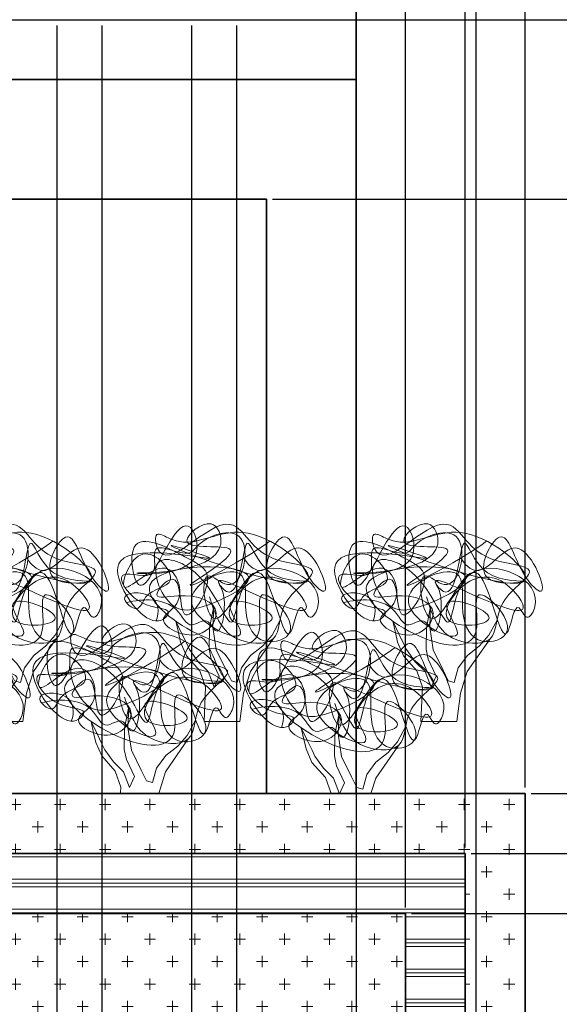
# Model space of a CAD drawing. Units: millimetres. Extents: x -692 to 9639, y -141 to 10345.
# Tile 8 of 19: x 7929 to 8831, y 1504 to 3148. Entities that reach past the tile are written whole.
import ezdxf

# ---------------------------------------------------------------- set-up
doc = ezdxf.new("R2010")
doc.units = ezdxf.units.MM
doc.header["$MEASUREMENT"] = 0
for name, color, linetype, lineweight in [('A-ANNO-DIMS', 2, 'Continuous', 18), ('A-ELEV', 7, 'Continuous', 35), ('A-ELEV-PATT', 8, 'Continuous', 13), ('L-PLNT', 3, 'Continuous', 18)]:
    doc.layers.add(name, color=color, linetype=linetype, lineweight=lineweight)
doc.styles.get("Standard").update_dxf_attribs({"font": 'arial.ttf'})
doc.dimstyles.get("Standard").update_dxf_attribs({"dimtxt": 25, "dimasz": 20, "dimexe": 0.18, "dimexo": 10, "dimgap": 10, "dimtad": 0, "dimtih": 1, "dimtoh": 1, "dimdec": 0, "dimzin": 0, "dimdsep": 46, "dimtxsty": 'Standard', "dimcen": 10, "dimadec": 0, "dimazin": 0, "dimtfac": 1, "dimtdec": 0, "dimtofl": 0, "dimtmove": 0, "dimatfit": 3, "dimfxl": 1, "dimtolj": 1, "dimtzin": 0, "dimarcsym": 0})

# ---------------------------------------------------------------- blocks, each defined once
blk = doc.blocks.new('SHRUB-A')
for p, q in [((56.2, 156.7), (63.1, 192.4)), ((63.1, 192.4), (61.6, 157.6)), ((4.3, 148.6), (0, 167.6)), ((0, 167.6), (10, 146.8)), ((160.6, 144.2), (174.3, 169.5)), ((7.9, 132.5), (4.3, 148.6)), ((55.6, 120.9), (56.2, 156.7)), ((61.6, 157.6), (67.3, 119.6)), ((17.8, 109.9), (7.9, 132.5)), ((10, 146.8), (18, 130.3)), ((162.4, 138.4), (124.4, 83.7)), ((145.1, 126.5), (160.6, 144.2)), ((18, 130.3), (22.9, 120.3)), ((22.9, 120.3), (37.4, 100.1)), ((59.1, 104.1), (55.6, 120.9)), ((67.3, 119.6), (83.9, 86)), ((124.8, 110.5), (145.1, 126.5)), ((40.2, 84.8), (17.8, 109.9)), ((37.4, 100.1), (54, 83.6)), ((72.4, 75.8), (59.1, 104.1)), ((109.4, 89.7), (124.8, 110.5)), ((49.7, 57.7), (40.2, 84.8)), ((54, 83.6), (64.1, 57.4)), ((83.9, 86), (92.7, 68.2)), ((102.6, 65.4), (109.4, 89.7)), ((124.4, 83.7), (113, 47.4)), ((64.1, 57.4), (72.4, 75.8)), ((92.7, 68.2), (102.6, 65.4)), ((47, 0.4), (49.7, 57.7)), ((113, 47.4), (106.7, 0)), ((106.7, 0), (47, 0.4))]:
    blk.add_line(p, q)
blk = doc.blocks.new('SHRUB-B')
for p, q in [((56.2, 99.2), (63.1, 135)), ((63.1, 135), (61.6, 100.2)), ((4.3, 91.2), (0, 110.2)), ((0, 110.2), (10, 89.4)), ((55.6, 63.5), (56.2, 99.2)), ((61.6, 100.2), (67.3, 62.2)), ((160.6, 86.8), (174.3, 112.1)), ((7.9, 75.1), (4.3, 91.2)), ((10, 89.4), (18, 72.9)), ((145.1, 69.1), (160.6, 86.8)), ((17.8, 52.5), (7.9, 75.1)), ((18, 72.9), (22.9, 62.9)), ((124.8, 53.1), (145.1, 69.1)), ((40.2, 27.4), (17.8, 52.5)), ((22.9, 62.9), (37.4, 42.7)), ((59.1, 46.7), (55.6, 63.5)), ((67.3, 62.2), (83.9, 28.6)), ((109.4, 32.3), (124.8, 53.1)), ((37.4, 42.7), (54, 26.2)), ((72.4, 18.4), (59.1, 46.7)), ((49.7, 0.3), (40.2, 27.4)), ((54, 26.2), (64.1, 0)), ((64.1, 0), (72.4, 18.4)), ((83.9, 28.6), (92.7, 10.8)), ((102.6, 8), (109.4, 32.3)), ((92.7, 10.8), (102.6, 8))]:
    blk.add_line(p, q)
blk = doc.blocks.new('*D7')
at = {"layer": 'A-ANNO-DIMS', "color": 0, "lineweight": -2, "transparency": 16777216}
for p, q in [((8481.5, 9848.8), (-649.1, 9848.8)), ((-648.9, 9828.8), (-648.9, 5124.9)), ((-648.9, 375.6), (-648.9, 5079.4)), ((2463.7, 355.6), (-649.1, 355.6))]:
    blk.add_line(p, q, dxfattribs=at)
at = {"layer": 'A-ANNO-DIMS', "color": 0, "lineweight": -3, "transparency": 16777216}
for points in [[(-652.2, 9828.8), (-645.6, 9828.8), (-648.9, 9848.8)], [(-652.2, 375.6), (-645.6, 375.6), (-648.9, 355.6)]]:
    blk.add_solid(points, dxfattribs=at)
at = {"layer": 'Defpoints', "color": 0, "lineweight": -3, "transparency": 16777216}
for p in [(-648.9, 9848.8), (8491.5, 9848.8), (2473.7, 355.6)]:
    blk.add_point(p, dxfattribs=at)
at = {"layer": 'A-ANNO-DIMS', "color": 0, "transparency": 16777216, "insert": (-648.9, 5102.2), "char_height": 25, "attachment_point": 5}
blk.add_mtext('\\A1;9493', dxfattribs=at)
blk = doc.blocks.new('*D9')
at = {"layer": 'A-ANNO-DIMS', "color": 0, "lineweight": -2, "transparency": 16777216}
for p, q in [((8501.5, 8848.8), (9553.9, 8848.8)), ((9553.7, 8828.8), (9553.7, 4874.9)), ((9553.7, 875.6), (9553.7, 4829.4)), ((9083.7, 855.6), (9553.9, 855.6))]:
    blk.add_line(p, q, dxfattribs=at)
at = {"layer": 'A-ANNO-DIMS', "color": 0, "lineweight": -3, "transparency": 16777216}
for points in [[(9550.4, 8828.8), (9557.1, 8828.8), (9553.7, 8848.8)], [(9550.4, 875.6), (9557.1, 875.6), (9553.7, 855.6)]]:
    blk.add_solid(points, dxfattribs=at)
at = {"layer": 'Defpoints', "color": 0, "lineweight": -3, "transparency": 16777216}
for p in [(8491.5, 8848.8), (9553.7, 8848.8), (9073.7, 855.6)]:
    blk.add_point(p, dxfattribs=at)
at = {"layer": 'A-ANNO-DIMS', "color": 0, "transparency": 16777216, "insert": (9553.7, 4852.2), "char_height": 25, "attachment_point": 5}
blk.add_mtext('\\A1;7993', dxfattribs=at)
blk = doc.blocks.new('*D28')
at = {"layer": 'A-ANNO-DIMS', "color": 0, "lineweight": -2, "transparency": 16777216}
for p, q in [((8583.7, 1655.6), (9553.9, 1655.6)), ((9553.7, 1635.6), (9553.7, 1278.3)), ((9553.7, 875.6), (9553.7, 1232.8)), ((8583.7, 855.6), (9553.9, 855.6))]:
    blk.add_line(p, q, dxfattribs=at)
at = {"layer": 'A-ANNO-DIMS', "color": 0, "lineweight": -3, "transparency": 16777216}
for points in [[(9550.4, 1635.6), (9557.1, 1635.6), (9553.7, 1655.6)], [(9550.4, 875.6), (9557.1, 875.6), (9553.7, 855.6)]]:
    blk.add_solid(points, dxfattribs=at)
at = {"layer": 'Defpoints', "color": 0, "lineweight": -3, "transparency": 16777216}
for p in [(8573.7, 1655.6), (9553.7, 1655.6), (8573.7, 855.6)]:
    blk.add_point(p, dxfattribs=at)
at = {"layer": 'A-ANNO-DIMS', "color": 0, "transparency": 16777216, "insert": (9553.7, 1255.6), "char_height": 25, "attachment_point": 5}
blk.add_mtext('\\A1;800', dxfattribs=at)
blk = doc.blocks.new('*D29')
at = {"layer": 'A-ANNO-DIMS', "color": 0, "lineweight": -2, "transparency": 16777216}
for p, q in [((9553.7, 1755.6), (9553.7, 1775.6)), ((9553.7, 1775.6), (9573.7, 1775.6)), ((8683.7, 1755.6), (9553.9, 1755.6)), ((9553.7, 1675.6), (9553.7, 1735.6)), ((8583.7, 1655.6), (9553.9, 1655.6))]:
    blk.add_line(p, q, dxfattribs=at)
at = {"layer": 'A-ANNO-DIMS', "color": 0, "lineweight": -3, "transparency": 16777216}
for points in [[(9550.4, 1735.6), (9557.1, 1735.6), (9553.7, 1755.6)], [(9550.4, 1675.6), (9557.1, 1675.6), (9553.7, 1655.6)]]:
    blk.add_solid(points, dxfattribs=at)
at = {"layer": 'Defpoints', "color": 0, "lineweight": -3, "transparency": 16777216}
for p in [(8673.7, 1755.6), (9553.7, 1755.6), (8573.7, 1655.6)]:
    blk.add_point(p, dxfattribs=at)
at = {"layer": 'A-ANNO-DIMS', "color": 0, "transparency": 16777216, "insert": (9610.1, 1775.6), "char_height": 25, "attachment_point": 5}
blk.add_mtext('\\A1;100', dxfattribs=at)
blk = doc.blocks.new('*D30')
at = {"layer": 'A-ANNO-DIMS', "color": 0, "lineweight": -2, "transparency": 16777216}
for p, q in [((9553.7, 1855.6), (9553.7, 1875.6)), ((9553.7, 1875.6), (9573.7, 1875.6)), ((8783.7, 1855.6), (9553.9, 1855.6)), ((9553.7, 1775.6), (9553.7, 1835.6)), ((8683.7, 1755.6), (9553.9, 1755.6))]:
    blk.add_line(p, q, dxfattribs=at)
at = {"layer": 'A-ANNO-DIMS', "color": 0, "lineweight": -3, "transparency": 16777216}
for points in [[(9550.4, 1835.6), (9557.1, 1835.6), (9553.7, 1855.6)], [(9550.4, 1775.6), (9557.1, 1775.6), (9553.7, 1755.6)]]:
    blk.add_solid(points, dxfattribs=at)
at = {"layer": 'Defpoints', "color": 0, "lineweight": -3, "transparency": 16777216}
for p in [(8773.7, 1855.6), (9553.7, 1855.6), (8673.7, 1755.6)]:
    blk.add_point(p, dxfattribs=at)
at = {"layer": 'A-ANNO-DIMS', "color": 0, "transparency": 16777216, "insert": (9610.1, 1875.6), "char_height": 25, "attachment_point": 5}
blk.add_mtext('\\A1;100', dxfattribs=at)
blk = doc.blocks.new('*D31')
at = {"layer": 'A-ANNO-DIMS', "color": 0, "lineweight": -2, "transparency": 16777216}
for p, q in [((8351.5, 2848.3), (9553.9, 2848.3)), ((9553.7, 2828.3), (9553.7, 2374.7)), ((9553.7, 1875.6), (9553.7, 2329.2)), ((8783.7, 1855.6), (9553.9, 1855.6))]:
    blk.add_line(p, q, dxfattribs=at)
at = {"layer": 'A-ANNO-DIMS', "color": 0, "lineweight": -3, "transparency": 16777216}
for points in [[(9550.4, 2828.3), (9557.1, 2828.3), (9553.7, 2848.3)], [(9550.4, 1875.6), (9557.1, 1875.6), (9553.7, 1855.6)]]:
    blk.add_solid(points, dxfattribs=at)
at = {"layer": 'Defpoints', "color": 0, "lineweight": -3, "transparency": 16777216}
for p in [(8341.5, 2848.3), (9553.7, 2848.3), (8773.7, 1855.6)]:
    blk.add_point(p, dxfattribs=at)
at = {"layer": 'A-ANNO-DIMS', "color": 0, "transparency": 16777216, "insert": (9553.7, 2351.9), "char_height": 25, "attachment_point": 5}
blk.add_mtext('\\A1;992.7', dxfattribs=at)
blk = doc.blocks.new('*D34')
at = {"layer": 'A-ANNO-DIMS', "color": 0, "lineweight": -2, "transparency": 16777216}
for p, q in [((7091.7, 1665.6), (7091.7, 10329)), ((7111.7, 10328.8), (7786.7, 10328.8)), ((8553.7, 10328.8), (7878.8, 10328.8)), ((8573.7, 1665.6), (8573.7, 10329))]:
    blk.add_line(p, q, dxfattribs=at)
at = {"layer": 'A-ANNO-DIMS', "color": 0, "lineweight": -3, "transparency": 16777216}
for points in [[(7111.7, 10332.1), (7111.7, 10325.4), (7091.7, 10328.8)], [(8553.7, 10332.1), (8553.7, 10325.4), (8573.7, 10328.8)]]:
    blk.add_solid(points, dxfattribs=at)
at = {"layer": 'Defpoints', "color": 0, "lineweight": -3, "transparency": 16777216}
for p in [(8573.7, 10328.8), (7091.7, 1655.6), (8573.7, 1655.6)]:
    blk.add_point(p, dxfattribs=at)
at = {"layer": 'A-ANNO-DIMS', "color": 0, "transparency": 16777216, "insert": (7832.7, 10328.8), "char_height": 25, "attachment_point": 5}
blk.add_mtext('\\A1;1482', dxfattribs=at)
blk = doc.blocks.new('*D35')
at = {"layer": 'A-ANNO-DIMS', "color": 0, "lineweight": -2, "transparency": 16777216}
for p, q in [((8553.7, 10328.8), (8533.7, 10328.8)), ((8573.7, 1665.6), (8573.7, 10329)), ((8673.7, 1765.6), (8673.7, 10329)), ((8693.7, 10328.8), (8713.7, 10328.8))]:
    blk.add_line(p, q, dxfattribs=at)
at = {"layer": 'A-ANNO-DIMS', "color": 0, "lineweight": -3, "transparency": 16777216}
for points in [[(8553.7, 10332.1), (8553.7, 10325.4), (8573.7, 10328.8)], [(8693.7, 10332.1), (8693.7, 10325.4), (8673.7, 10328.8)]]:
    blk.add_solid(points, dxfattribs=at)
at = {"layer": 'Defpoints', "color": 0, "lineweight": -3, "transparency": 16777216}
for p in [(8673.7, 10328.8), (8673.7, 1755.6), (8573.7, 1655.6)]:
    blk.add_point(p, dxfattribs=at)
at = {"layer": 'A-ANNO-DIMS', "color": 0, "transparency": 16777216, "insert": (8623.7, 10328.8), "char_height": 25, "attachment_point": 5}
blk.add_mtext('\\A1;100', dxfattribs=at)
blk = doc.blocks.new('*D36')
at = {"layer": 'A-ANNO-DIMS', "color": 0, "lineweight": -2, "transparency": 16777216}
for p, q in [((8653.7, 10328.8), (8633.7, 10328.8)), ((8673.7, 1765.6), (8673.7, 10329)), ((8773.7, 1865.6), (8773.7, 10329)), ((8793.7, 10328.8), (8813.7, 10328.8))]:
    blk.add_line(p, q, dxfattribs=at)
at = {"layer": 'A-ANNO-DIMS', "color": 0, "lineweight": -3, "transparency": 16777216}
for points in [[(8653.7, 10332.1), (8653.7, 10325.4), (8673.7, 10328.8)], [(8793.7, 10332.1), (8793.7, 10325.4), (8773.7, 10328.8)]]:
    blk.add_solid(points, dxfattribs=at)
at = {"layer": 'Defpoints', "color": 0, "lineweight": -3, "transparency": 16777216}
for p in [(8773.7, 10328.8), (8773.7, 1855.6), (8673.7, 1755.6)]:
    blk.add_point(p, dxfattribs=at)
at = {"layer": 'A-ANNO-DIMS', "color": 0, "transparency": 16777216, "insert": (8723.7, 10328.8), "char_height": 25, "attachment_point": 5}
blk.add_mtext('\\A1;100', dxfattribs=at)
blk = doc.blocks.new('*D46')
at = {"layer": 'A-ANNO-DIMS', "color": 0, "lineweight": -2, "transparency": 16777216}
for p, q in [((7841.5, 3138.3), (7841.5, -124.6)), ((7991.5, 3138.3), (7991.5, -124.6)), ((7861.5, -124.4), (7880.1, -124.4)), ((7971.5, -124.4), (7952.9, -124.4))]:
    blk.add_line(p, q, dxfattribs=at)
at = {"layer": 'A-ANNO-DIMS', "color": 0, "lineweight": -3, "transparency": 16777216}
for points in [[(7861.5, -121.1), (7861.5, -127.8), (7841.5, -124.4)], [(7971.5, -121.1), (7971.5, -127.8), (7991.5, -124.4)]]:
    blk.add_solid(points, dxfattribs=at)
at = {"layer": 'Defpoints', "color": 0, "lineweight": -3, "transparency": 16777216}
for p in [(7841.5, 3148.3), (7991.5, 3148.3), (7991.5, -124.4)]:
    blk.add_point(p, dxfattribs=at)
at = {"layer": 'A-ANNO-DIMS', "color": 0, "transparency": 16777216, "insert": (7916.5, -124.4), "char_height": 25, "attachment_point": 5}
blk.add_mtext('\\A1;150', dxfattribs=at)
blk = doc.blocks.new('*D47')
at = {"layer": 'A-ANNO-DIMS', "color": 0, "lineweight": -2, "transparency": 16777216}
for p, q in [((7991.5, 3138.3), (7991.5, -124.6)), ((8066.5, 3138.3), (8066.5, -124.6)), ((8011.5, -124.4), (8046.5, -124.4)), ((8066.5, -124.4), (8086.5, -124.4))]:
    blk.add_line(p, q, dxfattribs=at)
at = {"layer": 'A-ANNO-DIMS', "color": 0, "lineweight": -3, "transparency": 16777216}
for points in [[(8011.5, -121.1), (8011.5, -127.8), (7991.5, -124.4)], [(8046.5, -121.1), (8046.5, -127.8), (8066.5, -124.4)]]:
    blk.add_solid(points, dxfattribs=at)
at = {"layer": 'Defpoints', "color": 0, "lineweight": -3, "transparency": 16777216}
for p in [(7991.5, 3148.3), (8066.5, 3148.3), (8066.5, -124.4)]:
    blk.add_point(p, dxfattribs=at)
at = {"layer": 'A-ANNO-DIMS', "color": 0, "transparency": 16777216, "insert": (8114.4, -124.4), "char_height": 25, "attachment_point": 5}
blk.add_mtext('\\A1;75', dxfattribs=at)
blk = doc.blocks.new('*D48')
at = {"layer": 'A-ANNO-DIMS', "color": 0, "lineweight": -2, "transparency": 16777216}
for p, q in [((8066.5, 3138.3), (8066.5, -124.6)), ((8216.5, 3138.3), (8216.5, -124.6)), ((8086.5, -124.4), (8105.1, -124.4)), ((8196.5, -124.4), (8177.9, -124.4))]:
    blk.add_line(p, q, dxfattribs=at)
at = {"layer": 'A-ANNO-DIMS', "color": 0, "lineweight": -3, "transparency": 16777216}
for points in [[(8086.5, -121.1), (8086.5, -127.8), (8066.5, -124.4)], [(8196.5, -121.1), (8196.5, -127.8), (8216.5, -124.4)]]:
    blk.add_solid(points, dxfattribs=at)
at = {"layer": 'Defpoints', "color": 0, "lineweight": -3, "transparency": 16777216}
for p in [(8066.5, 3148.3), (8216.5, 3148.3), (8216.5, -124.4)]:
    blk.add_point(p, dxfattribs=at)
at = {"layer": 'A-ANNO-DIMS', "color": 0, "transparency": 16777216, "insert": (8141.5, -124.4), "char_height": 25, "attachment_point": 5}
blk.add_mtext('\\A1;150', dxfattribs=at)
blk = doc.blocks.new('*D49')
at = {"layer": 'A-ANNO-DIMS', "color": 0, "lineweight": -2, "transparency": 16777216}
for p, q in [((8216.5, 3138.3), (8216.5, -124.6)), ((8291.5, 3138.3), (8291.5, -124.6)), ((8236.5, -124.4), (8271.5, -124.4)), ((8291.5, -124.4), (8311.5, -124.4))]:
    blk.add_line(p, q, dxfattribs=at)
at = {"layer": 'A-ANNO-DIMS', "color": 0, "lineweight": -3, "transparency": 16777216}
for points in [[(8236.5, -121.1), (8236.5, -127.8), (8216.5, -124.4)], [(8271.5, -121.1), (8271.5, -127.8), (8291.5, -124.4)]]:
    blk.add_solid(points, dxfattribs=at)
at = {"layer": 'Defpoints', "color": 0, "lineweight": -3, "transparency": 16777216}
for p in [(8216.5, 3148.3), (8291.5, 3148.3), (8291.5, -124.4)]:
    blk.add_point(p, dxfattribs=at)
at = {"layer": 'A-ANNO-DIMS', "color": 0, "transparency": 16777216, "insert": (8339.4, -124.4), "char_height": 25, "attachment_point": 5}
blk.add_mtext('\\A1;75', dxfattribs=at)
blk = doc.blocks.new('*D50')
at = {"layer": 'A-ANNO-DIMS', "color": 0, "lineweight": -2, "transparency": 16777216}
for p, q in [((8291.5, 3138.3), (8291.5, -124.6)), ((8491.5, 3138.3), (8491.5, -124.6)), ((8311.5, -124.4), (8353.8, -124.4)), ((8471.5, -124.4), (8429.3, -124.4))]:
    blk.add_line(p, q, dxfattribs=at)
at = {"layer": 'A-ANNO-DIMS', "color": 0, "lineweight": -3, "transparency": 16777216}
for points in [[(8311.5, -121.1), (8311.5, -127.8), (8291.5, -124.4)], [(8471.5, -121.1), (8471.5, -127.8), (8491.5, -124.4)]]:
    blk.add_solid(points, dxfattribs=at)
at = {"layer": 'Defpoints', "color": 0, "lineweight": -3, "transparency": 16777216}
for p in [(8291.5, 3148.3), (8491.5, 3148.3), (8491.5, -124.4)]:
    blk.add_point(p, dxfattribs=at)
at = {"layer": 'A-ANNO-DIMS', "color": 0, "transparency": 16777216, "insert": (8391.5, -124.4), "char_height": 25, "attachment_point": 5}
blk.add_mtext('\\A1;200', dxfattribs=at)
blk = doc.blocks.new('*D51')
at = {"layer": 'A-ANNO-DIMS', "color": 0, "lineweight": -2, "transparency": 16777216}
for p, q in [((8691.5, 4838.8), (8691.5, -124.6)), ((8491.5, 3138.3), (8491.5, -124.6)), ((8511.5, -124.4), (8553.8, -124.4)), ((8671.5, -124.4), (8629.3, -124.4))]:
    blk.add_line(p, q, dxfattribs=at)
at = {"layer": 'A-ANNO-DIMS', "color": 0, "lineweight": -3, "transparency": 16777216}
for points in [[(8511.5, -121.1), (8511.5, -127.8), (8491.5, -124.4)], [(8671.5, -121.1), (8671.5, -127.8), (8691.5, -124.4)]]:
    blk.add_solid(points, dxfattribs=at)
at = {"layer": 'Defpoints', "color": 0, "lineweight": -3, "transparency": 16777216}
for p in [(8691.5, 4848.8), (8491.5, 3148.3), (8691.5, -124.4)]:
    blk.add_point(p, dxfattribs=at)
at = {"layer": 'A-ANNO-DIMS', "color": 0, "transparency": 16777216, "insert": (8591.5, -124.4), "char_height": 25, "attachment_point": 5}
blk.add_mtext('\\A1;200', dxfattribs=at)
blk = doc.blocks.new('*D71')
at = {"layer": 'A-ANNO-DIMS', "color": 0, "lineweight": -2, "transparency": 16777216}
for p, q in [((5201.5, 3598.3), (9553.9, 3598.3)), ((9553.7, 3578.3), (9553.7, 3396)), ((9553.7, 3168.3), (9553.7, 3350.5)), ((5101.5, 3148.3), (9553.9, 3148.3))]:
    blk.add_line(p, q, dxfattribs=at)
at = {"layer": 'A-ANNO-DIMS', "color": 0, "lineweight": -3, "transparency": 16777216}
for points in [[(9550.4, 3578.3), (9557.1, 3578.3), (9553.7, 3598.3)], [(9550.4, 3168.3), (9557.1, 3168.3), (9553.7, 3148.3)]]:
    blk.add_solid(points, dxfattribs=at)
at = {"layer": 'Defpoints', "color": 0, "lineweight": -3, "transparency": 16777216}
for p in [(5191.5, 3598.3), (9553.7, 3598.3), (5091.5, 3148.3)]:
    blk.add_point(p, dxfattribs=at)
at = {"layer": 'A-ANNO-DIMS', "color": 0, "transparency": 16777216, "insert": (9553.7, 3373.3), "char_height": 25, "attachment_point": 5}
blk.add_mtext('\\A1;450', dxfattribs=at)

msp = doc.modelspace()

# ---------------------------------------------------------------- hatches: boundary and pattern name
at = {"layer": 'A-ELEV-PATT'}
h = msp.add_hatch(dxfattribs=at)
h.set_pattern_fill('CROSS', color=256, scale=150)
h.paths.add_polyline_path([(8573.746, 1655.575), (7091.746, 1655.575), (7091.746, 855.575), (7273.746, 855.575), (8573.746, 855.575)], flags=17)
h.paths.add_polyline_path([(8773.746, 1855.575), (8463.966, 1855.575), (8463.828, 1855.268), (8463.709, 1855.575), (7761.103, 1855.575), (7760.965, 1855.268), (7760.846, 1855.575), (7409.705, 1855.575), (7409.567, 1855.268), (7409.448, 1855.575), (7076.174, 1855.575), (7076.035, 1855.268), (7075.916, 1855.575), (6891.746, 1855.575), (6891.746, 855.575), (6991.746, 855.575), (6991.746, 1755.575), (8673.746, 1755.575), (8673.746, 855.575), (8773.746, 855.575)])
h = msp.add_hatch(dxfattribs=at)
h.set_pattern_fill('PLAST', color=256, scale=200)
h.paths.add_polyline_path([(8673.746, 1755.575), (6991.746, 1755.575), (6991.746, 855.575), (7091.746, 855.575), (7091.746, 1655.575), (8573.746, 1655.575), (8573.746, 855.575), (8673.746, 855.575)])

# ---------------------------------------------------------------- linework, layer by layer
at = {"layer": 'A-ELEV'}
for p, q in [((8491.547, 4848.772), (8491.547, 1855.575)), ((5191.547, 3048.27), (8491.547, 3048.27)), ((5773.746, 2848.27), (8341.547, 2848.27)), ((8341.547, 2848.27), (8341.547, 1855.575)), ((8773.746, 1855.575), (6891.746, 1855.575)), ((8773.746, 1855.575), (8773.746, 855.575)), ((8673.746, 1755.575), (6991.746, 1755.575)), ((8673.746, 1755.575), (8673.746, 855.575)), ((8573.746, 1655.575), (7091.746, 1655.575)), ((8573.746, 1655.575), (8573.746, 855.575))]:
    msp.add_line(p, q, dxfattribs=at)
at = {"layer": 'L-PLNT'}
for p, q in [((8104.579, 1965.211), (8111.567, 2000.918)), ((8111.567, 2000.918), (8110.002, 1966.165)), ((8052.702, 1957.134), (8048.428, 1976.125)), ((8048.428, 1976.125), (8058.469, 1955.382)), ((8208.984, 1952.778), (8222.715, 1978.029)), ((8056.315, 1941.086), (8052.702, 1957.134)), ((8104.023, 1929.473), (8104.579, 1965.211)), ((8110.002, 1966.165), (8115.774, 1928.138)), ((8066.226, 1918.461), (8056.315, 1941.086)), ((8058.469, 1955.382), (8066.458, 1938.88)), ((8210.873, 1946.937), (8172.808, 1892.206)), ((8193.491, 1935.076), (8208.984, 1952.778)), ((8066.458, 1938.88), (8071.29, 1928.899)), ((8071.29, 1928.899), (8085.863, 1908.658)), ((8107.495, 1912.661), (8104.023, 1929.473)), ((8115.774, 1928.138), (8132.332, 1894.515)), ((8173.193, 1919.065), (8193.491, 1935.076)), ((8562.132, 1936.243), (8524.067, 1881.512)), ((8088.612, 1893.382), (8066.226, 1918.461)), ((8085.863, 1908.658), (8102.421, 1892.113)), ((8120.848, 1884.375), (8107.495, 1912.661)), ((8157.83, 1898.301), (8173.193, 1919.065)), ((8098.109, 1866.269), (8088.612, 1893.382)), ((8102.421, 1892.113), (8112.569, 1865.962)), ((8132.332, 1894.515), (8141.082, 1876.748)), ((8151.027, 1873.967), (8157.83, 1898.301)), ((8172.808, 1892.206), (8161.459, 1856.004)), ((8112.569, 1865.962), (8120.848, 1884.375)), ((8141.082, 1876.748), (8151.027, 1873.967)), ((8524.067, 1881.512), (8516.49, 1857.344)), ((8097.695, 1857.344), (8098.109, 1866.269))]:
    msp.add_line(p, q, dxfattribs=at)
for points, knots in [([(7941.428, 2249.042), (7947.933, 2237.706), (7981.169, 2207.754), (8037.599, 2319.362), (8096.779, 2167.67), (8032.143, 2229.166), (8016.418, 2328.371), (7949.459, 2194.758), (8086.925, 2215.079), (7970.08, 2204.712), (7940.744, 2329.754), (7935.142, 2163.076), (7882.64, 2224.979), (7976.321, 2179.391), (8073.386, 2141.303), (8004.226, 2230.619), (7938.072, 2210.89), (7895.861, 2127.262), (8046.749, 2141.658), (7881.14, 2203.471), (7977.514, 2083.661), (7783.672, 2177.336), (7958.368, 2256.385), (7936.159, 2158.211), (7964.897, 2098.948), (8051.149, 2123.83), (7949.315, 2228.342), (8004.521, 2029.162), (7618.927, 2240.289), (8034.021, 2243.554), (7884.038, 2166.62), (7813.186, 2156.226), (7770.374, 2264.065), (7885.155, 2230.339), (7927.243, 2085.9), (7932.228, 2275.464), (8093.922, 2209.432), (8051.195, 2140.066), (8033.158, 2187.643), (8012.363, 2051.748), (7975.609, 2333.663), (7888.478, 2070.375), (7863.476, 2246.68), (7933.245, 2175.732), (7964.912, 2316.142), (7874.371, 2285.782), (7845.246, 2244.752), (7778.303, 2291.151), (7804.494, 2204.577), (7712.052, 2240.713), (7761.869, 2161.604), (7823.388, 2165.76), (7793.222, 2127.131), (7737.918, 2181.977), (7713.636, 2288.868), (7958.01, 2226.655), (7709.719, 2307.83), (8170.468, 2128.857), (7944.803, 2328.1), (7864.96, 2267.378), (7818.657, 2280.064), (7790.573, 2295.919), (7802.935, 2206.055), (7904.263, 2346.33), (7956.403, 2266.58), (7995.218, 2241.096), (8086.893, 2233.207), (7993.877, 2180.878), (8008.037, 2100.111), (7908.22, 2108.211), (7892.593, 2156.893), (7883.85, 2184.132)], [2413.81083439, 2413.81083439, 2413.81083439, 2413.81083439, 2446.13175162, 2525.76080664, 2606.35842411, 2641.00152553, 2720.74212251, 2790.99014926, 2851.81652626, 2913.32865241, 2976.26621652, 3063.90114016, 3082.75198237, 3142.42040078, 3234.21047015, 3290.89514405, 3366.44484787, 3415.98940505, 3483.69911772, 3557.93307926, 3609.73318023, 3705.73947781, 3799.4035149, 3865.9559372, 3923.0506034, 3967.47996902, 4044.49288828, 4106.44083814, 4304.51898163, 4470.20683119, 4567.66187689, 4605.3795614, 4686.71522755, 4750.59418277, 4853.67923318, 4940.38216709, 5061.92671957, 5081.75583403, 5102.38342504, 5145.20608443, 5257.20859169, 5364.77120979, 5434.601162, 5468.93345211, 5548.91442162, 5624.29444335, 5636.24531967, 5696.20028889, 5735.53268567, 5783.76480276, 5846.42206129, 5886.03768999, 5892.5373904, 5975.51315878, 6025.10951571, 6171.93373357, 6229.50952465, 6457.88730992, 6585.61219414, 6694.59236697, 6720.94216912, 6740.48817363, 6762.80712224, 6890.45590486, 6938.76737224, 6996.52597549, 7050.2147859, 7119.04318667, 7183.57042671, 7247.02609863, 7327.63038966, 7327.63038966, 7327.63038966, 7327.63038966]), ([(7794.737, 2143.94), (7800.8, 2158.144), (7797.305, 2196.249), (7722.734, 2191.386), (7766.182, 2154.108), (7776.863, 2198.183), (7845.924, 2201.259), (7765.972, 2293.571), (7717.477, 2156.7), (7815.952, 2271.959), (7847.727, 2174.361), (7783.674, 2143.553), (7866.477, 2102.288), (7913.823, 2169.843), (7849.377, 2193.667), (7778.836, 2176.214), (7840.34, 2245.325), (7827.395, 2104.492), (7901.707, 2221.171), (7835.943, 2254.125), (7740.167, 2308.243), (7764.333, 2163.685), (7803.906, 2260.33), (7851.043, 2324.908), (7884.633, 2215.034), (7655.885, 2230.018), (7930.034, 2217.011), (7890.032, 2326.244), (7806.634, 2255.543), (7981.668, 2284.242), (7770.144, 2159.222), (7934.397, 2239.906), (7984.529, 2277.481)], [369.05069933, 369.05069933, 369.05069933, 369.05069933, 408.0755152, 451.81999766, 477.70991819, 501.76804774, 551.72688153, 614.71506468, 677.59190345, 752.65992621, 814.92518896, 848.06947292, 911.78367098, 957.89252981, 1028.01014559, 1063.15062915, 1099.93333455, 1162.00574744, 1235.23981988, 1278.45742209, 1371.86548038, 1434.47491944, 1513.90135623, 1562.79289697, 1613.81915843, 1716.27616866, 1864.9556669, 1902.31221643, 1951.61463942, 2025.20033993, 2111.30740148, 2244.75178922, 2244.75178922, 2244.75178922, 2244.75178922]), ([(8303.871, 2249.042), (8310.377, 2237.706), (8343.613, 2207.754), (8400.043, 2319.362), (8459.223, 2167.67), (8394.587, 2229.166), (8378.861, 2328.371), (8311.902, 2194.758), (8449.368, 2215.079), (8332.524, 2204.712), (8303.188, 2329.754), (8297.585, 2163.076), (8245.084, 2224.979), (8338.764, 2179.391), (8435.83, 2141.303), (8366.669, 2230.619), (8300.516, 2210.89), (8258.305, 2127.262), (8409.192, 2141.658), (8243.583, 2203.471), (8339.958, 2083.661), (8146.116, 2177.336), (8320.812, 2256.385), (8298.603, 2158.211), (8327.34, 2098.948), (8413.593, 2123.83), (8311.759, 2228.342), (8366.965, 2029.162), (7981.371, 2240.289), (8396.465, 2243.554), (8246.482, 2166.62), (8175.63, 2156.226), (8132.817, 2264.065), (8247.598, 2230.339), (8289.686, 2085.9), (8294.672, 2275.464), (8456.365, 2209.432), (8413.638, 2140.066), (8395.601, 2187.643), (8374.806, 2051.748), (8338.053, 2333.663), (8250.921, 2070.375), (8225.919, 2246.68), (8295.688, 2175.732), (8327.355, 2316.142), (8236.815, 2285.782), (8207.689, 2244.752), (8140.747, 2291.151), (8166.938, 2204.577), (8074.496, 2240.713), (8124.312, 2161.604), (8185.832, 2165.76), (8155.665, 2127.131), (8100.361, 2181.977), (8076.08, 2288.868), (8320.454, 2226.655), (8072.162, 2307.83), (8532.911, 2128.857), (8307.247, 2328.1), (8227.403, 2267.378), (8181.101, 2280.064), (8153.017, 2295.919), (8165.379, 2206.055), (8266.707, 2346.33), (8318.847, 2266.58), (8357.661, 2241.096), (8449.337, 2233.207), (8356.32, 2180.878), (8370.481, 2100.111), (8270.663, 2108.211), (8255.037, 2156.893), (8246.293, 2184.132)], [2413.81083439, 2413.81083439, 2413.81083439, 2413.81083439, 2446.13175162, 2525.76080664, 2606.35842411, 2641.00152553, 2720.74212251, 2790.99014926, 2851.81652626, 2913.32865241, 2976.26621652, 3063.90114016, 3082.75198237, 3142.42040078, 3234.21047015, 3290.89514405, 3366.44484787, 3415.98940505, 3483.69911772, 3557.93307926, 3609.73318023, 3705.73947781, 3799.4035149, 3865.9559372, 3923.0506034, 3967.47996902, 4044.49288828, 4106.44083814, 4304.51898163, 4470.20683119, 4567.66187689, 4605.3795614, 4686.71522755, 4750.59418277, 4853.67923318, 4940.38216709, 5061.92671957, 5081.75583403, 5102.38342504, 5145.20608443, 5257.20859169, 5364.77120979, 5434.601162, 5468.93345211, 5548.91442162, 5624.29444335, 5636.24531967, 5696.20028889, 5735.53268567, 5783.76480276, 5846.42206129, 5886.03768999, 5892.5373904, 5975.51315878, 6025.10951571, 6171.93373357, 6229.50952465, 6457.88730992, 6585.61219414, 6694.59236697, 6720.94216912, 6740.48817363, 6762.80712224, 6890.45590486, 6938.76737224, 6996.52597549, 7050.2147859, 7119.04318667, 7183.57042671, 7247.02609863, 7327.63038966, 7327.63038966, 7327.63038966, 7327.63038966]), ([(8157.18, 2143.94), (8163.243, 2158.144), (8159.749, 2196.249), (8085.177, 2191.386), (8128.625, 2154.108), (8139.307, 2198.183), (8208.368, 2201.259), (8128.416, 2293.571), (8079.92, 2156.7), (8178.396, 2271.959), (8210.171, 2174.361), (8146.118, 2143.553), (8228.92, 2102.288), (8276.267, 2169.843), (8211.821, 2193.667), (8141.279, 2176.214), (8202.784, 2245.325), (8189.839, 2104.492), (8264.151, 2221.171), (8198.387, 2254.125), (8102.611, 2308.243), (8126.776, 2163.685), (8166.35, 2260.33), (8213.486, 2324.908), (8247.077, 2215.034), (8018.329, 2230.018), (8292.478, 2217.011), (8252.476, 2326.244), (8169.077, 2255.543), (8344.112, 2284.242), (8132.588, 2159.222), (8296.841, 2239.906), (8346.972, 2277.481)], [369.05069933, 369.05069933, 369.05069933, 369.05069933, 408.0755152, 451.81999766, 477.70991819, 501.76804774, 551.72688153, 614.71506468, 677.59190345, 752.65992621, 814.92518896, 848.06947292, 911.78367098, 957.89252981, 1028.01014559, 1063.15062915, 1099.93333455, 1162.00574744, 1235.23981988, 1278.45742209, 1371.86548038, 1434.47491944, 1513.90135623, 1562.79289697, 1613.81915843, 1716.27616866, 1864.9556669, 1902.31221643, 1951.61463942, 2025.20033993, 2111.30740148, 2244.75178922, 2244.75178922, 2244.75178922, 2244.75178922]), ([(8666.315, 2249.042), (8672.821, 2237.706), (8706.056, 2207.754), (8762.486, 2319.362), (8821.667, 2167.67), (8757.03, 2229.166), (8741.305, 2328.371), (8674.346, 2194.758), (8811.812, 2215.079), (8694.967, 2204.712), (8665.631, 2329.754), (8660.029, 2163.076), (8607.527, 2224.979), (8701.208, 2179.391), (8798.274, 2141.303), (8729.113, 2230.619), (8662.959, 2210.89), (8620.748, 2127.262), (8771.636, 2141.658), (8606.027, 2203.471), (8702.401, 2083.661), (8508.559, 2177.336), (8683.255, 2256.385), (8661.047, 2158.211), (8689.784, 2098.948), (8776.036, 2123.83), (8674.202, 2228.342), (8729.408, 2029.162), (8343.815, 2240.289), (8758.908, 2243.554), (8608.925, 2166.62), (8538.073, 2156.226), (8495.261, 2264.065), (8610.042, 2230.339), (8652.13, 2085.9), (8657.115, 2275.464), (8818.809, 2209.432), (8776.082, 2140.066), (8758.045, 2187.643), (8737.25, 2051.748), (8700.496, 2333.663), (8613.365, 2070.375), (8588.363, 2246.68), (8658.132, 2175.732), (8689.799, 2316.142), (8599.258, 2285.782), (8570.133, 2244.752), (8503.19, 2291.151), (8529.381, 2204.577), (8436.939, 2240.713), (8486.756, 2161.604), (8548.276, 2165.76), (8518.109, 2127.131), (8462.805, 2181.977), (8438.523, 2288.868), (8682.898, 2226.655), (8434.606, 2307.83), (8895.355, 2128.857), (8669.69, 2328.1), (8589.847, 2267.378), (8543.544, 2280.064), (8515.46, 2295.919), (8527.822, 2206.055), (8629.151, 2346.33), (8681.29, 2266.58), (8720.105, 2241.096), (8811.781, 2233.207), (8718.764, 2180.878), (8732.925, 2100.111), (8633.107, 2108.211), (8617.48, 2156.893), (8608.737, 2184.132)], [2413.81083439, 2413.81083439, 2413.81083439, 2413.81083439, 2446.13175162, 2525.76080664, 2606.35842411, 2641.00152553, 2720.74212251, 2790.99014926, 2851.81652626, 2913.32865241, 2976.26621652, 3063.90114016, 3082.75198237, 3142.42040078, 3234.21047015, 3290.89514405, 3366.44484787, 3415.98940505, 3483.69911772, 3557.93307926, 3609.73318023, 3705.73947781, 3799.4035149, 3865.9559372, 3923.0506034, 3967.47996902, 4044.49288828, 4106.44083814, 4304.51898163, 4470.20683119, 4567.66187689, 4605.3795614, 4686.71522755, 4750.59418277, 4853.67923318, 4940.38216709, 5061.92671957, 5081.75583403, 5102.38342504, 5145.20608443, 5257.20859169, 5364.77120979, 5434.601162, 5468.93345211, 5548.91442162, 5624.29444335, 5636.24531967, 5696.20028889, 5735.53268567, 5783.76480276, 5846.42206129, 5886.03768999, 5892.5373904, 5975.51315878, 6025.10951571, 6171.93373357, 6229.50952465, 6457.88730992, 6585.61219414, 6694.59236697, 6720.94216912, 6740.48817363, 6762.80712224, 6890.45590486, 6938.76737224, 6996.52597549, 7050.2147859, 7119.04318667, 7183.57042671, 7247.02609863, 7327.63038966, 7327.63038966, 7327.63038966, 7327.63038966]), ([(8519.624, 2143.94), (8525.687, 2158.144), (8522.192, 2196.249), (8447.621, 2191.386), (8491.069, 2154.108), (8501.75, 2198.183), (8570.811, 2201.259), (8490.859, 2293.571), (8442.364, 2156.7), (8540.839, 2271.959), (8572.615, 2174.361), (8508.561, 2143.553), (8591.364, 2102.288), (8638.711, 2169.843), (8574.264, 2193.667), (8503.723, 2176.214), (8565.227, 2245.325), (8552.283, 2104.492), (8626.594, 2221.171), (8560.83, 2254.125), (8465.055, 2308.243), (8489.22, 2163.685), (8528.793, 2260.33), (8575.93, 2324.908), (8609.521, 2215.034), (8380.773, 2230.018), (8654.921, 2217.011), (8614.92, 2326.244), (8531.521, 2255.543), (8706.555, 2284.242), (8495.031, 2159.222), (8659.285, 2239.906), (8709.416, 2277.481)], [369.05069933, 369.05069933, 369.05069933, 369.05069933, 408.0755152, 451.81999766, 477.70991819, 501.76804774, 551.72688153, 614.71506468, 677.59190345, 752.65992621, 814.92518896, 848.06947292, 911.78367098, 957.89252981, 1028.01014559, 1063.15062915, 1099.93333455, 1162.00574744, 1235.23981988, 1278.45742209, 1371.86548038, 1434.47491944, 1513.90135623, 1562.79289697, 1613.81915843, 1716.27616866, 1864.9556669, 1902.31221643, 1951.61463942, 2025.20033993, 2111.30740148, 2244.75178922, 2244.75178922, 2244.75178922, 2244.75178922]), ([(8261.901, 2206.874), (8265.391, 2200.207), (8276.888, 2178.247), (8263.817, 2104.319), (8242.636, 2153.752), (8209.825, 2125.304), (8192.239, 2181.552), (8134.486, 2182.208), (8107.774, 2174.344)], [0, 0, 0, 0, 24.87287104, 81.92705424, 103.09014331, 128.64171207, 165.87657864, 231.33124244, 231.33124244, 231.33124244, 231.33124244]), ([(8624.344, 2206.874), (8627.835, 2200.207), (8639.331, 2178.247), (8626.26, 2104.319), (8605.079, 2153.752), (8572.269, 2125.304), (8554.682, 2181.552), (8496.929, 2182.208), (8470.218, 2174.344)], [0, 0, 0, 0, 24.87287104, 81.92705424, 103.09014331, 128.64171207, 165.87657864, 231.33124244, 231.33124244, 231.33124244, 231.33124244]), ([(8162.096, 2081.693), (8168.601, 2070.358), (8201.837, 2040.406), (8258.267, 2152.014), (8317.447, 2000.321), (8252.811, 2061.817), (8237.086, 2161.023), (8170.127, 2027.41), (8307.593, 2047.73), (8190.748, 2037.363), (8161.412, 2162.405), (8155.81, 1995.728), (8103.308, 2057.63), (8196.989, 2012.042), (8294.055, 1973.955), (8224.894, 2063.27), (8158.74, 2043.541), (8116.529, 1959.913), (8267.417, 1974.309), (8101.808, 2036.122), (8198.182, 1916.312), (8004.34, 2009.987), (8179.036, 2089.036), (8156.828, 1990.863), (8185.565, 1931.599), (8271.817, 1956.482), (8169.983, 2060.993), (8225.189, 1861.813), (7839.595, 2072.94), (8254.689, 2076.205), (8104.706, 1999.271), (8033.854, 1988.878), (7991.042, 2096.717), (8105.823, 2062.99), (8147.911, 1918.551), (8152.896, 2108.116), (8314.59, 2042.083), (8271.863, 1972.717), (8253.826, 2020.295), (8233.031, 1884.399), (8196.277, 2166.314), (8109.146, 1903.027), (8084.144, 2079.331), (8153.913, 2008.384), (8185.58, 2148.793), (8095.039, 2118.434), (8065.914, 2077.403), (7998.971, 2123.803), (8025.162, 2037.228), (7932.72, 2073.364), (7982.537, 1994.255), (8044.056, 1998.412), (8013.89, 1959.783), (7958.586, 2014.628), (7934.304, 2121.519), (8178.679, 2059.306), (7930.387, 2140.481), (8391.136, 1961.508), (8165.471, 2160.751), (8085.628, 2100.029), (8039.325, 2112.716), (8011.241, 2128.571), (8023.603, 2038.706), (8124.932, 2178.981), (8177.071, 2099.231), (8215.886, 2073.747), (8307.562, 2065.858), (8214.545, 2013.53), (8228.705, 1932.762), (8128.888, 1940.862), (8113.261, 1989.545), (8104.518, 2016.783)], [2413.81083439, 2413.81083439, 2413.81083439, 2413.81083439, 2446.13175162, 2525.76080664, 2606.35842411, 2641.00152553, 2720.74212251, 2790.99014926, 2851.81652626, 2913.32865241, 2976.26621652, 3063.90114016, 3082.75198237, 3142.42040078, 3234.21047015, 3290.89514405, 3366.44484787, 3415.98940505, 3483.69911772, 3557.93307926, 3609.73318023, 3705.73947781, 3799.4035149, 3865.9559372, 3923.0506034, 3967.47996902, 4044.49288828, 4106.44083814, 4304.51898163, 4470.20683119, 4567.66187689, 4605.3795614, 4686.71522755, 4750.59418277, 4853.67923318, 4940.38216709, 5061.92671957, 5081.75583403, 5102.38342504, 5145.20608443, 5257.20859169, 5364.77120979, 5434.601162, 5468.93345211, 5548.91442162, 5624.29444335, 5636.24531967, 5696.20028889, 5735.53268567, 5783.76480276, 5846.42206129, 5886.03768999, 5892.5373904, 5975.51315878, 6025.10951571, 6171.93373357, 6229.50952465, 6457.88730992, 6585.61219414, 6694.59236697, 6720.94216912, 6740.48817363, 6762.80712224, 6890.45590486, 6938.76737224, 6996.52597549, 7050.2147859, 7119.04318667, 7183.57042671, 7247.02609863, 7327.63038966, 7327.63038966, 7327.63038966, 7327.63038966]), ([(8015.405, 1976.591), (8021.468, 1990.795), (8017.973, 2028.9), (7943.402, 2024.038), (7986.85, 1986.759), (7997.531, 2030.834), (8066.592, 2033.911), (7986.64, 2126.222), (7938.145, 1989.352), (8036.62, 2104.61), (8068.395, 2007.013), (8004.342, 1976.204), (8087.145, 1934.94), (8134.491, 2002.494), (8070.045, 2026.318), (7999.504, 2008.866), (8061.008, 2077.976), (8048.064, 1937.143), (8122.375, 2053.823), (8056.611, 2086.776), (7960.836, 2140.895), (7985.001, 1996.336), (8024.574, 2092.982), (8071.711, 2157.56), (8105.302, 2047.686), (7876.554, 2062.669), (8150.702, 2049.663), (8110.701, 2158.895), (8027.302, 2088.194), (8202.336, 2116.894), (7990.812, 1991.873), (8155.065, 2072.558), (8205.197, 2110.133)], [369.05069933, 369.05069933, 369.05069933, 369.05069933, 408.0755152, 451.81999766, 477.70991819, 501.76804774, 551.72688153, 614.71506468, 677.59190345, 752.65992621, 814.92518896, 848.06947292, 911.78367098, 957.89252981, 1028.01014559, 1063.15062915, 1099.93333455, 1162.00574744, 1235.23981988, 1278.45742209, 1371.86548038, 1434.47491944, 1513.90135623, 1562.79289697, 1613.81915843, 1716.27616866, 1864.9556669, 1902.31221643, 1951.61463942, 2025.20033993, 2111.30740148, 2244.75178922, 2244.75178922, 2244.75178922, 2244.75178922]), ([(7810.492, 2070.999), (7816.997, 2059.664), (7850.233, 2029.712), (7906.663, 2141.319), (7965.843, 1989.627), (7901.207, 2051.123), (7885.481, 2150.328), (7818.522, 2016.716), (7955.988, 2037.036), (7839.144, 2026.669), (7809.808, 2151.711), (7804.206, 1985.034), (7751.704, 2046.936), (7845.385, 2001.348), (7942.45, 1963.26), (7873.289, 2052.576), (7807.136, 2032.847), (7764.925, 1949.219), (7915.813, 1963.615), (7750.204, 2025.428), (7846.578, 1905.618), (7652.736, 1999.293), (7827.432, 2078.342), (7805.223, 1980.168), (7833.961, 1920.905), (7920.213, 1945.788), (7818.379, 2050.299), (7873.585, 1851.119), (7487.991, 2062.246), (7903.085, 2065.511), (7753.102, 1988.577), (7682.25, 1978.184), (7639.438, 2086.023), (7754.219, 2052.296), (7796.307, 1907.857), (7801.292, 2097.422), (7962.985, 2031.389), (7920.258, 1962.023), (7902.221, 2009.601), (7881.426, 1873.705), (7844.673, 2155.62), (7757.542, 1892.333), (7732.54, 2068.637), (7802.309, 1997.689), (7833.975, 2138.099), (7743.435, 2107.74), (7714.309, 2066.709), (7647.367, 2113.109), (7673.558, 2026.534), (7581.116, 2062.67), (7630.933, 1983.561), (7692.452, 1987.717), (7662.286, 1949.089), (7606.982, 2003.934), (7582.7, 2110.825), (7827.074, 2048.612), (7578.782, 2129.787), (8039.532, 1950.814), (7813.867, 2150.057), (7734.023, 2089.335), (7687.721, 2102.021), (7659.637, 2117.876), (7671.999, 2028.012), (7773.327, 2168.287), (7825.467, 2088.537), (7864.281, 2063.053), (7955.957, 2055.164), (7862.94, 2002.836), (7877.101, 1922.068), (7777.284, 1930.168), (7761.657, 1978.85), (7752.914, 2006.089)], [2413.81083439, 2413.81083439, 2413.81083439, 2413.81083439, 2446.13175162, 2525.76080664, 2606.35842411, 2641.00152553, 2720.74212251, 2790.99014926, 2851.81652626, 2913.32865241, 2976.26621652, 3063.90114016, 3082.75198237, 3142.42040078, 3234.21047015, 3290.89514405, 3366.44484787, 3415.98940505, 3483.69911772, 3557.93307926, 3609.73318023, 3705.73947781, 3799.4035149, 3865.9559372, 3923.0506034, 3967.47996902, 4044.49288828, 4106.44083814, 4304.51898163, 4470.20683119, 4567.66187689, 4605.3795614, 4686.71522755, 4750.59418277, 4853.67923318, 4940.38216709, 5061.92671957, 5081.75583403, 5102.38342504, 5145.20608443, 5257.20859169, 5364.77120979, 5434.601162, 5468.93345211, 5548.91442162, 5624.29444335, 5636.24531967, 5696.20028889, 5735.53268567, 5783.76480276, 5846.42206129, 5886.03768999, 5892.5373904, 5975.51315878, 6025.10951571, 6171.93373357, 6229.50952465, 6457.88730992, 6585.61219414, 6694.59236697, 6720.94216912, 6740.48817363, 6762.80712224, 6890.45590486, 6938.76737224, 6996.52597549, 7050.2147859, 7119.04318667, 7183.57042671, 7247.02609863, 7327.63038966, 7327.63038966, 7327.63038966, 7327.63038966]), ([(8513.355, 2070.999), (8519.86, 2059.664), (8553.096, 2029.712), (8609.526, 2141.319), (8668.706, 1989.627), (8604.07, 2051.123), (8588.345, 2150.328), (8521.386, 2016.716), (8658.852, 2037.036), (8542.007, 2026.669), (8512.671, 2151.711), (8507.069, 1985.034), (8454.567, 2046.936), (8548.248, 2001.348), (8645.313, 1963.26), (8576.153, 2052.576), (8509.999, 2032.847), (8467.788, 1949.219), (8618.676, 1963.615), (8453.067, 2025.428), (8549.441, 1905.618), (8355.599, 1999.293), (8530.295, 2078.342), (8508.086, 1980.168), (8536.824, 1920.905), (8623.076, 1945.788), (8521.242, 2050.299), (8576.448, 1851.119), (8190.854, 2062.246), (8605.948, 2065.511), (8455.965, 1988.577), (8385.113, 1978.184), (8342.301, 2086.023), (8457.082, 2052.296), (8499.17, 1907.857), (8504.155, 2097.422), (8665.849, 2031.389), (8623.122, 1962.023), (8605.084, 2009.601), (8584.29, 1873.705), (8547.536, 2155.62), (8460.405, 1892.333), (8435.403, 2068.637), (8505.172, 1997.689), (8536.839, 2138.099), (8446.298, 2107.74), (8417.172, 2066.709), (8350.23, 2113.109), (8376.421, 2026.534), (8283.979, 2062.67), (8333.796, 1983.561), (8395.315, 1987.717), (8365.149, 1949.089), (8309.845, 2003.934), (8285.563, 2110.825), (8529.937, 2048.612), (8281.646, 2129.787), (8742.395, 1950.814), (8516.73, 2150.057), (8436.887, 2089.335), (8390.584, 2102.021), (8362.5, 2117.876), (8374.862, 2028.012), (8476.19, 2168.287), (8528.33, 2088.537), (8567.145, 2063.053), (8658.82, 2055.164), (8565.804, 2002.836), (8579.964, 1922.068), (8480.147, 1930.168), (8464.52, 1978.85), (8455.777, 2006.089)], [2413.81083439, 2413.81083439, 2413.81083439, 2413.81083439, 2446.13175162, 2525.76080664, 2606.35842411, 2641.00152553, 2720.74212251, 2790.99014926, 2851.81652626, 2913.32865241, 2976.26621652, 3063.90114016, 3082.75198237, 3142.42040078, 3234.21047015, 3290.89514405, 3366.44484787, 3415.98940505, 3483.69911772, 3557.93307926, 3609.73318023, 3705.73947781, 3799.4035149, 3865.9559372, 3923.0506034, 3967.47996902, 4044.49288828, 4106.44083814, 4304.51898163, 4470.20683119, 4567.66187689, 4605.3795614, 4686.71522755, 4750.59418277, 4853.67923318, 4940.38216709, 5061.92671957, 5081.75583403, 5102.38342504, 5145.20608443, 5257.20859169, 5364.77120979, 5434.601162, 5468.93345211, 5548.91442162, 5624.29444335, 5636.24531967, 5696.20028889, 5735.53268567, 5783.76480276, 5846.42206129, 5886.03768999, 5892.5373904, 5975.51315878, 6025.10951571, 6171.93373357, 6229.50952465, 6457.88730992, 6585.61219414, 6694.59236697, 6720.94216912, 6740.48817363, 6762.80712224, 6890.45590486, 6938.76737224, 6996.52597549, 7050.2147859, 7119.04318667, 7183.57042671, 7247.02609863, 7327.63038966, 7327.63038966, 7327.63038966, 7327.63038966]), ([(8366.664, 1965.897), (8372.727, 1980.101), (8369.232, 2018.206), (8294.661, 2013.343), (8338.109, 1976.065), (8348.79, 2020.14), (8417.851, 2023.217), (8337.899, 2115.528), (8289.404, 1978.657), (8387.879, 2093.916), (8419.654, 1996.319), (8355.601, 1965.51), (8438.404, 1924.245), (8485.75, 1991.8), (8421.304, 2015.624), (8350.763, 1998.171), (8412.267, 2067.282), (8399.322, 1926.449), (8473.634, 2043.128), (8407.87, 2076.082), (8312.094, 2130.201), (8336.26, 1985.642), (8375.833, 2082.287), (8422.97, 2146.866), (8456.56, 2036.992), (8227.812, 2051.975), (8501.961, 2038.969), (8461.959, 2148.201), (8378.56, 2077.5), (8553.595, 2106.199), (8342.071, 1981.179), (8506.324, 2061.864), (8556.456, 2099.439)], [369.05069933, 369.05069933, 369.05069933, 369.05069933, 408.0755152, 451.81999766, 477.70991819, 501.76804774, 551.72688153, 614.71506468, 677.59190345, 752.65992621, 814.92518896, 848.06947292, 911.78367098, 957.89252981, 1028.01014559, 1063.15062915, 1099.93333455, 1162.00574744, 1235.23981988, 1278.45742209, 1371.86548038, 1434.47491944, 1513.90135623, 1562.79289697, 1613.81915843, 1716.27616866, 1864.9556669, 1902.31221643, 1951.61463942, 2025.20033993, 2111.30740148, 2244.75178922, 2244.75178922, 2244.75178922, 2244.75178922]), ([(8120.125, 2039.526), (8123.616, 2032.859), (8135.112, 2010.899), (8122.041, 1936.97), (8100.86, 1986.404), (8068.05, 1957.955), (8050.463, 2014.203), (7992.71, 2014.86), (7965.999, 2006.996)], [0, 0, 0, 0, 24.87287104, 81.92705424, 103.09014331, 128.64171207, 165.87657864, 231.33124244, 231.33124244, 231.33124244, 231.33124244]), ([(8471.384, 2028.831), (8474.874, 2022.164), (8486.371, 2000.205), (8473.3, 1926.276), (8452.119, 1975.71), (8419.309, 1947.261), (8401.722, 2003.509), (8343.969, 2004.166), (8317.258, 1996.302)], [0, 0, 0, 0, 24.87287104, 81.92705424, 103.09014331, 128.64171207, 165.87657864, 231.33124244, 231.33124244, 231.33124244, 231.33124244])]:
    msp.add_open_spline(points, degree=3, knots=knots, dxfattribs=at)

# ---------------------------------------------------------------- block references
for name, p in [('SHRUB-A', (7827.759, 1975.903)), ('SHRUB-A', (8190.203, 1975.903)), ('SHRUB-A', (8552.647, 1975.903)), ('SHRUB-B', (8399.687, 1855.268))]:
    msp.add_blockref(name, p, dxfattribs=at)

# ---------------------------------------------------------------- dimensions: what is measured, and where the dimension line sits
at = {"layer": 'A-ANNO-DIMS'}
for base, p1, p2, picture, middle in [((8573.746, 10328.772), (7091.746, 1655.575), (8573.746, 1655.575), '*D34', (7832.746, 10328.772)), ((8673.746, 10328.772), (8573.746, 1655.575), (8673.746, 1755.575), '*D35', (8623.746, 10328.772)), ((8773.746, 10328.772), (8673.746, 1755.575), (8773.746, 1855.575), '*D36', (8723.746, 10328.772)), ((8691.547, -124.425), (8491.547, 3148.27), (8691.547, 4848.772), '*D51', (8591.547, -124.425)), ((7991.547, -124.425), (7841.547, 3148.27), (7991.547, 3148.27), '*D46', (7916.547, -124.425)), ((8066.547, -124.425), (7991.547, 3148.27), (8066.547, 3148.27), '*D47', (8114.444, -124.425)), ((8216.547, -124.425), (8066.547, 3148.27), (8216.547, 3148.27), '*D48', (8141.547, -124.425)), ((8291.547, -124.425), (8216.547, 3148.27), (8291.547, 3148.27), '*D49', (8339.444, -124.425)), ((8491.547, -124.425), (8291.547, 3148.27), (8491.547, 3148.27), '*D50', (8391.547, -124.425))]:
    dim = msp.add_linear_dim(base=base, p1=p1, p2=p2, dimstyle='Standard', override={"dimdec": 0, "dimlfac": 1, "dimrnd": 0, "dimzin": 0, "dimdsep": 46, "dimlunit": 2}, dxfattribs=at)
    dim.commit()
    dim.dimension.update_dxf_attribs({"geometry": picture, "text_midpoint": middle})
for base, p1, p2, override, picture, middle in [((-648.912, 9848.772), (2473.746, 355.575), (8491.547, 9848.772), {"dimdec": 0, "dimlfac": 1, "dimrnd": 0, "dimzin": 0, "dimdsep": 46, "dimlunit": 2}, '*D7', (-648.912, 5102.173)), ((9553.746, 8848.772), (9073.746, 855.575), (8491.547, 8848.772), {"dimdec": 0, "dimlfac": 1, "dimrnd": 0, "dimzin": 0, "dimdsep": 46, "dimlunit": 2}, '*D9', (9553.746, 4852.173)), ((9553.746, 3598.27), (5091.547, 3148.27), (5191.547, 3598.27), {"dimdec": 0, "dimlfac": 1, "dimrnd": 0, "dimzin": 0, "dimdsep": 46, "dimlunit": 2}, '*D71', (9553.746, 3373.27)), ((9553.746, 2848.27), (8773.746, 1855.575), (8341.547, 2848.27), {"dimdec": 1, "dimlfac": 1, "dimrnd": 0, "dimzin": 0, "dimdsep": 46, "dimlunit": 2}, '*D31', (9553.746, 2351.922)), ((9553.746, 1855.575), (8673.746, 1755.575), (8773.746, 1855.575), {"dimdec": 0, "dimlfac": 1, "dimrnd": 0, "dimzin": 0, "dimdsep": 46, "dimlunit": 2}, '*D30', (9610.144, 1875.575)), ((9553.746, 1755.575), (8573.746, 1655.575), (8673.746, 1755.575), {"dimdec": 0, "dimlfac": 1, "dimrnd": 0, "dimzin": 0, "dimdsep": 46, "dimlunit": 2}, '*D29', (9610.144, 1775.575)), ((9553.746, 1655.575), (8573.746, 855.575), (8573.746, 1655.575), {"dimdec": 0, "dimlfac": 1, "dimrnd": 0, "dimzin": 0, "dimdsep": 46, "dimlunit": 2}, '*D28', (9553.746, 1255.575))]:
    dim = msp.add_linear_dim(base=base, p1=p1, p2=p2, angle=90, dimstyle='Standard', override=override, dxfattribs=at)
    dim.commit()
    dim.dimension.update_dxf_attribs({"geometry": picture, "text_midpoint": middle})

doc.saveas('drawing.dxf')
